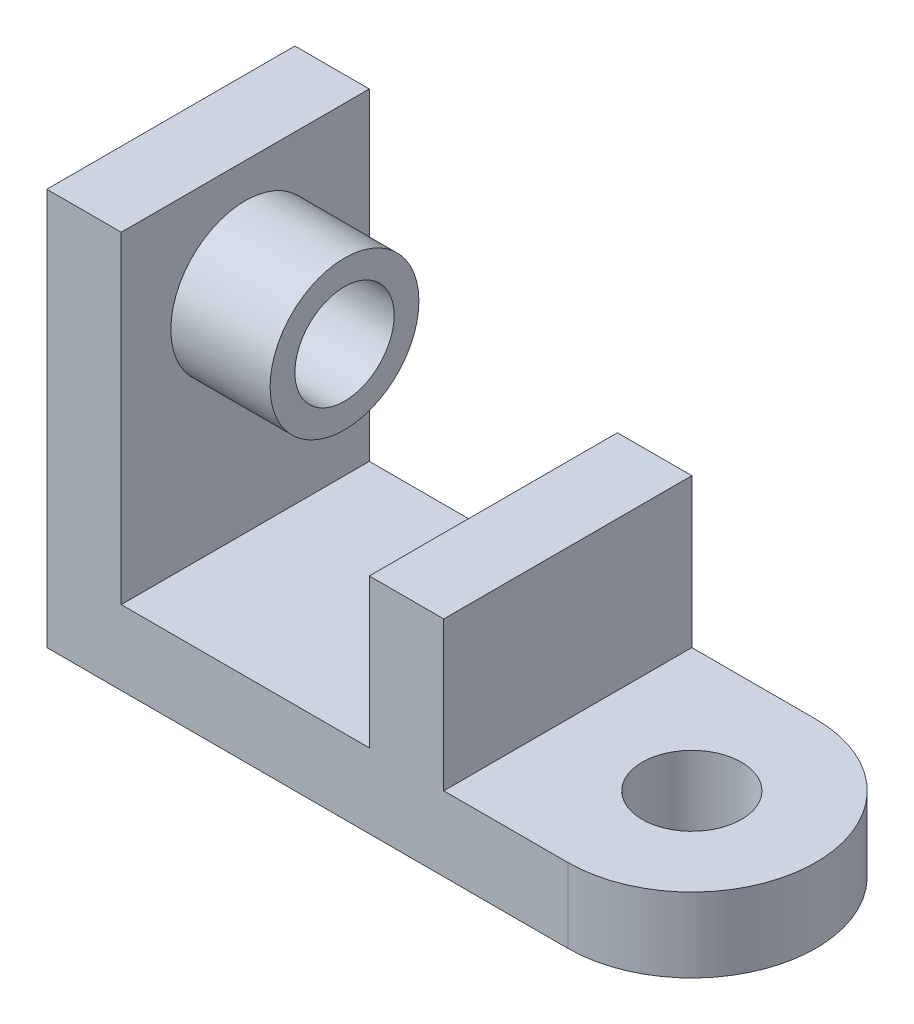
ISO-10303-21;
HEADER;
FILE_DESCRIPTION(('STEP AP214'),'2;1');
FILE_NAME('part.step','',(''),(''),'','','');
FILE_SCHEMA(('AUTOMOTIVE_DESIGN { 1 0 10303 214 1 1 1 1 }'));
ENDSEC;
DATA;
#1=APPLICATION_CONTEXT('core data for automotive mechanical design processes');
#2=APPLICATION_PROTOCOL_DEFINITION('international standard','automotive_design',2000,#1);
#3=PRODUCT_CONTEXT('',#1,'mechanical');
#4=PRODUCT('Part','Part','',(#3));
#5=PRODUCT_RELATED_PRODUCT_CATEGORY('part','',(#4));
#6=PRODUCT_DEFINITION_FORMATION('','',#4);
#7=PRODUCT_DEFINITION_CONTEXT('part definition',#1,'design');
#8=PRODUCT_DEFINITION('design','',#6,#7);
#9=PRODUCT_DEFINITION_SHAPE('','',#8);
#10=(LENGTH_UNIT() NAMED_UNIT(*) SI_UNIT(.MILLI.,.METRE.));
#11=(NAMED_UNIT(*) PLANE_ANGLE_UNIT() SI_UNIT($,.RADIAN.));
#12=(NAMED_UNIT(*) SI_UNIT($,.STERADIAN.) SOLID_ANGLE_UNIT());
#13=UNCERTAINTY_MEASURE_WITH_UNIT(LENGTH_MEASURE(1.E-05),#10,'distance_accuracy_value','');
#14=(GEOMETRIC_REPRESENTATION_CONTEXT(3) GLOBAL_UNCERTAINTY_ASSIGNED_CONTEXT((#13)) GLOBAL_UNIT_ASSIGNED_CONTEXT((#10,
#11,#12)) REPRESENTATION_CONTEXT('',''));
#15=CARTESIAN_POINT('',(0.,0.,0.));
#16=DIRECTION('',(0.,0.,1.));
#17=DIRECTION('',(1.,0.,0.));
#18=AXIS2_PLACEMENT_3D('',#15,#16,#17);
#19=CARTESIAN_POINT('',(40.,15.,0.));
#20=DIRECTION('',(0.,1.,0.));
#21=DIRECTION('',(0.,0.,1.));
#22=AXIS2_PLACEMENT_3D('',#19,#20,#21);
#23=PLANE('',#22);
#24=DIRECTION('',(1.,0.,0.));
#25=VECTOR('',#24,1.);
#26=CARTESIAN_POINT('',(-65.,15.,25.));
#27=LINE('',#26,#25);
#28=CARTESIAN_POINT('',(-50.,15.,25.));
#29=VERTEX_POINT('',#28);
#30=CARTESIAN_POINT('',(0.,15.,25.));
#31=VERTEX_POINT('',#30);
#32=EDGE_CURVE('E175',#29,#31,#27,.T.);
#33=ORIENTED_EDGE('',*,*,#32,.T.);
#34=DIRECTION('',(0.,0.,1.));
#35=VECTOR('',#34,1.);
#36=CARTESIAN_POINT('',(0.,15.,25.));
#37=LINE('',#36,#35);
#38=CARTESIAN_POINT('',(0.,15.,-25.));
#39=VERTEX_POINT('',#38);
#40=EDGE_CURVE('E223',#39,#31,#37,.T.);
#41=ORIENTED_EDGE('',*,*,#40,.F.);
#42=DIRECTION('',(-1.,0.,0.));
#43=VECTOR('',#42,1.);
#44=CARTESIAN_POINT('',(-65.,15.,-25.));
#45=LINE('',#44,#43);
#46=CARTESIAN_POINT('',(-50.,15.,-25.));
#47=VERTEX_POINT('',#46);
#48=EDGE_CURVE('E141',#39,#47,#45,.T.);
#49=ORIENTED_EDGE('',*,*,#48,.T.);
#50=DIRECTION('',(0.,0.,-1.));
#51=VECTOR('',#50,1.);
#52=CARTESIAN_POINT('',(-50.,15.,25.));
#53=LINE('',#52,#51);
#54=EDGE_CURVE('E65',#29,#47,#53,.T.);
#55=ORIENTED_EDGE('',*,*,#54,.F.);
#56=EDGE_LOOP('',(#33,#41,#49,#55));
#57=FACE_BOUND('',#56,.T.);
#58=ADVANCED_FACE('F41',(#57),#23,.T.);
#59=CARTESIAN_POINT('',(40.,15.,0.));
#60=DIRECTION('',(0.,1.,0.));
#61=DIRECTION('',(0.,0.,1.));
#62=AXIS2_PLACEMENT_3D('',#59,#60,#61);
#63=CIRCLE('',#62,10.);
#64=CARTESIAN_POINT('',(40.,15.,10.));
#65=VERTEX_POINT('',#64);
#66=EDGE_CURVE('E230',#65,#65,#63,.T.);
#67=ORIENTED_EDGE('',*,*,#66,.F.);
#68=EDGE_LOOP('',(#67));
#69=FACE_BOUND('',#68,.T.);
#70=CARTESIAN_POINT('',(40.,15.,-25.));
#71=VERTEX_POINT('',#70);
#72=CARTESIAN_POINT('',(15.,15.,-25.));
#73=VERTEX_POINT('',#72);
#74=EDGE_CURVE('E180',#71,#73,#45,.T.);
#75=ORIENTED_EDGE('',*,*,#74,.T.);
#76=DIRECTION('',(0.,0.,-1.));
#77=VECTOR('',#76,1.);
#78=CARTESIAN_POINT('',(15.,15.,-25.));
#79=LINE('',#78,#77);
#80=CARTESIAN_POINT('',(15.,15.,25.));
#81=VERTEX_POINT('',#80);
#82=EDGE_CURVE('E137',#81,#73,#79,.T.);
#83=ORIENTED_EDGE('',*,*,#82,.F.);
#84=CARTESIAN_POINT('',(40.,15.,25.));
#85=VERTEX_POINT('',#84);
#86=EDGE_CURVE('E179',#81,#85,#27,.T.);
#87=ORIENTED_EDGE('',*,*,#86,.T.);
#88=CARTESIAN_POINT('',(40.,15.,0.));
#89=DIRECTION('',(0.,1.,0.));
#90=DIRECTION('',(0.,0.,1.));
#91=AXIS2_PLACEMENT_3D('',#88,#89,#90);
#92=CIRCLE('',#91,25.);
#93=EDGE_CURVE('E178',#85,#71,#92,.T.);
#94=ORIENTED_EDGE('',*,*,#93,.T.);
#95=EDGE_LOOP('',(#75,#83,#87,#94));
#96=FACE_BOUND('',#95,.T.);
#97=ADVANCED_FACE('F217',(#69,#96),#23,.T.);
#98=CARTESIAN_POINT('',(-65.,15.,25.));
#99=DIRECTION('',(1.,0.,0.));
#100=DIRECTION('',(0.,0.,-1.));
#101=AXIS2_PLACEMENT_3D('',#98,#99,#100);
#102=PLANE('',#101);
#103=DIRECTION('',(0.,0.,1.));
#104=VECTOR('',#103,1.);
#105=CARTESIAN_POINT('',(-65.,0.,25.));
#106=LINE('',#105,#104);
#107=CARTESIAN_POINT('',(-65.,0.,-25.));
#108=VERTEX_POINT('',#107);
#109=CARTESIAN_POINT('',(-65.,0.,25.));
#110=VERTEX_POINT('',#109);
#111=EDGE_CURVE('E172',#108,#110,#106,.T.);
#112=ORIENTED_EDGE('',*,*,#111,.T.);
#113=DIRECTION('',(0.,-1.,0.));
#114=VECTOR('',#113,1.);
#115=CARTESIAN_POINT('',(-65.,15.,25.));
#116=LINE('',#115,#114);
#117=CARTESIAN_POINT('',(-65.,80.,25.));
#118=VERTEX_POINT('',#117);
#119=EDGE_CURVE('E47',#118,#110,#116,.T.);
#120=ORIENTED_EDGE('',*,*,#119,.F.);
#121=DIRECTION('',(0.,0.,1.));
#122=VECTOR('',#121,1.);
#123=CARTESIAN_POINT('',(-65.,80.,25.));
#124=LINE('',#123,#122);
#125=CARTESIAN_POINT('',(-65.,80.,-25.));
#126=VERTEX_POINT('',#125);
#127=EDGE_CURVE('E160',#126,#118,#124,.T.);
#128=ORIENTED_EDGE('',*,*,#127,.F.);
#129=DIRECTION('',(0.,-1.,0.));
#130=VECTOR('',#129,1.);
#131=CARTESIAN_POINT('',(-65.,15.,-25.));
#132=LINE('',#131,#130);
#133=EDGE_CURVE('E185',#126,#108,#132,.T.);
#134=ORIENTED_EDGE('',*,*,#133,.T.);
#135=EDGE_LOOP('',(#112,#120,#128,#134));
#136=FACE_BOUND('',#135,.T.);
#137=ADVANCED_FACE('F43',(#136),#102,.F.);
#138=CARTESIAN_POINT('',(-65.,15.,25.));
#139=DIRECTION('',(0.,0.,-1.));
#140=DIRECTION('',(-1.,0.,0.));
#141=AXIS2_PLACEMENT_3D('',#138,#139,#140);
#142=PLANE('',#141);
#143=DIRECTION('',(1.,0.,0.));
#144=VECTOR('',#143,1.);
#145=CARTESIAN_POINT('',(-65.,0.,25.));
#146=LINE('',#145,#144);
#147=CARTESIAN_POINT('',(40.,0.,25.));
#148=VERTEX_POINT('',#147);
#149=EDGE_CURVE('E183',#110,#148,#146,.T.);
#150=ORIENTED_EDGE('',*,*,#149,.T.);
#151=DIRECTION('',(0.,-1.,0.));
#152=VECTOR('',#151,1.);
#153=CARTESIAN_POINT('',(40.,15.,25.));
#154=LINE('',#153,#152);
#155=EDGE_CURVE('E198',#85,#148,#154,.T.);
#156=ORIENTED_EDGE('',*,*,#155,.F.);
#157=ORIENTED_EDGE('',*,*,#86,.F.);
#158=DIRECTION('',(0.,-1.,0.));
#159=VECTOR('',#158,1.);
#160=CARTESIAN_POINT('',(15.,45.,25.));
#161=LINE('',#160,#159);
#162=CARTESIAN_POINT('',(15.,45.,25.));
#163=VERTEX_POINT('',#162);
#164=EDGE_CURVE('E57',#163,#81,#161,.T.);
#165=ORIENTED_EDGE('',*,*,#164,.F.);
#166=DIRECTION('',(1.,0.,0.));
#167=VECTOR('',#166,1.);
#168=CARTESIAN_POINT('',(15.,45.,25.));
#169=LINE('',#168,#167);
#170=CARTESIAN_POINT('',(0.,45.,25.));
#171=VERTEX_POINT('',#170);
#172=EDGE_CURVE('E129',#171,#163,#169,.T.);
#173=ORIENTED_EDGE('',*,*,#172,.F.);
#174=DIRECTION('',(0.,-1.,0.));
#175=VECTOR('',#174,1.);
#176=CARTESIAN_POINT('',(0.,45.,25.));
#177=LINE('',#176,#175);
#178=EDGE_CURVE('E127',#171,#31,#177,.T.);
#179=ORIENTED_EDGE('',*,*,#178,.T.);
#180=ORIENTED_EDGE('',*,*,#32,.F.);
#181=DIRECTION('',(0.,-1.,0.));
#182=VECTOR('',#181,1.);
#183=CARTESIAN_POINT('',(-50.,80.,25.));
#184=LINE('',#183,#182);
#185=CARTESIAN_POINT('',(-50.,80.,25.));
#186=VERTEX_POINT('',#185);
#187=EDGE_CURVE('E168',#186,#29,#184,.T.);
#188=ORIENTED_EDGE('',*,*,#187,.F.);
#189=DIRECTION('',(1.,0.,0.));
#190=VECTOR('',#189,1.);
#191=CARTESIAN_POINT('',(-65.,80.,25.));
#192=LINE('',#191,#190);
#193=EDGE_CURVE('E159',#118,#186,#192,.T.);
#194=ORIENTED_EDGE('',*,*,#193,.F.);
#195=ORIENTED_EDGE('',*,*,#119,.T.);
#196=EDGE_LOOP('',(#150,#156,#157,#165,#173,#179,#180,#188,#194,#195));
#197=FACE_BOUND('',#196,.T.);
#198=ADVANCED_FACE('F203',(#197),#142,.F.);
#199=CARTESIAN_POINT('',(40.,15.,0.));
#200=DIRECTION('',(0.,-1.,0.));
#201=DIRECTION('',(0.,0.,-1.));
#202=AXIS2_PLACEMENT_3D('',#199,#200,#201);
#203=CYLINDRICAL_SURFACE('',#202,25.);
#204=CARTESIAN_POINT('',(40.,0.,0.));
#205=DIRECTION('',(0.,1.,0.));
#206=DIRECTION('',(0.,0.,1.));
#207=AXIS2_PLACEMENT_3D('',#204,#205,#206);
#208=CIRCLE('',#207,25.);
#209=CARTESIAN_POINT('',(40.,0.,-25.));
#210=VERTEX_POINT('',#209);
#211=EDGE_CURVE('E189',#148,#210,#208,.T.);
#212=ORIENTED_EDGE('',*,*,#211,.T.);
#213=DIRECTION('',(0.,-1.,0.));
#214=VECTOR('',#213,1.);
#215=CARTESIAN_POINT('',(40.,15.,-25.));
#216=LINE('',#215,#214);
#217=EDGE_CURVE('E192',#71,#210,#216,.T.);
#218=ORIENTED_EDGE('',*,*,#217,.F.);
#219=ORIENTED_EDGE('',*,*,#93,.F.);
#220=ORIENTED_EDGE('',*,*,#155,.T.);
#221=EDGE_LOOP('',(#212,#218,#219,#220));
#222=FACE_BOUND('',#221,.T.);
#223=ADVANCED_FACE('F213',(#222),#203,.T.);
#224=CARTESIAN_POINT('',(-65.,15.,-25.));
#225=DIRECTION('',(0.,0.,1.));
#226=DIRECTION('',(1.,0.,0.));
#227=AXIS2_PLACEMENT_3D('',#224,#225,#226);
#228=PLANE('',#227);
#229=DIRECTION('',(-1.,0.,0.));
#230=VECTOR('',#229,1.);
#231=CARTESIAN_POINT('',(-65.,0.,-25.));
#232=LINE('',#231,#230);
#233=EDGE_CURVE('E190',#210,#108,#232,.T.);
#234=ORIENTED_EDGE('',*,*,#233,.T.);
#235=ORIENTED_EDGE('',*,*,#133,.F.);
#236=DIRECTION('',(-1.,0.,0.));
#237=VECTOR('',#236,1.);
#238=CARTESIAN_POINT('',(-65.,80.,-25.));
#239=LINE('',#238,#237);
#240=CARTESIAN_POINT('',(-50.,80.,-25.));
#241=VERTEX_POINT('',#240);
#242=EDGE_CURVE('E163',#241,#126,#239,.T.);
#243=ORIENTED_EDGE('',*,*,#242,.F.);
#244=DIRECTION('',(0.,-1.,0.));
#245=VECTOR('',#244,1.);
#246=CARTESIAN_POINT('',(-50.,80.,-25.));
#247=LINE('',#246,#245);
#248=EDGE_CURVE('E170',#241,#47,#247,.T.);
#249=ORIENTED_EDGE('',*,*,#248,.T.);
#250=ORIENTED_EDGE('',*,*,#48,.F.);
#251=DIRECTION('',(0.,-1.,0.));
#252=VECTOR('',#251,1.);
#253=CARTESIAN_POINT('',(0.,45.,-25.));
#254=LINE('',#253,#252);
#255=CARTESIAN_POINT('',(0.,45.,-25.));
#256=VERTEX_POINT('',#255);
#257=EDGE_CURVE('E122',#256,#39,#254,.T.);
#258=ORIENTED_EDGE('',*,*,#257,.F.);
#259=DIRECTION('',(-1.,0.,0.));
#260=VECTOR('',#259,1.);
#261=CARTESIAN_POINT('',(0.,45.,-25.));
#262=LINE('',#261,#260);
#263=CARTESIAN_POINT('',(15.,45.,-25.));
#264=VERTEX_POINT('',#263);
#265=EDGE_CURVE('E128',#264,#256,#262,.T.);
#266=ORIENTED_EDGE('',*,*,#265,.F.);
#267=DIRECTION('',(0.,-1.,0.));
#268=VECTOR('',#267,1.);
#269=CARTESIAN_POINT('',(15.,45.,-25.));
#270=LINE('',#269,#268);
#271=EDGE_CURVE('E216',#264,#73,#270,.T.);
#272=ORIENTED_EDGE('',*,*,#271,.T.);
#273=ORIENTED_EDGE('',*,*,#74,.F.);
#274=ORIENTED_EDGE('',*,*,#217,.T.);
#275=EDGE_LOOP('',(#234,#235,#243,#249,#250,#258,#266,#272,#273,#274));
#276=FACE_BOUND('',#275,.T.);
#277=ADVANCED_FACE('F143',(#276),#228,.F.);
#278=CARTESIAN_POINT('',(40.,0.,0.));
#279=DIRECTION('',(0.,1.,0.));
#280=DIRECTION('',(0.,0.,1.));
#281=AXIS2_PLACEMENT_3D('',#278,#279,#280);
#282=PLANE('',#281);
#283=CARTESIAN_POINT('',(40.,0.,0.));
#284=DIRECTION('',(0.,1.,0.));
#285=DIRECTION('',(0.,0.,1.));
#286=AXIS2_PLACEMENT_3D('',#283,#284,#285);
#287=CIRCLE('',#286,10.);
#288=CARTESIAN_POINT('',(40.,0.,10.));
#289=VERTEX_POINT('',#288);
#290=EDGE_CURVE('E229',#289,#289,#287,.T.);
#291=ORIENTED_EDGE('',*,*,#290,.T.);
#292=EDGE_LOOP('',(#291));
#293=FACE_BOUND('',#292,.T.);
#294=ORIENTED_EDGE('',*,*,#111,.F.);
#295=ORIENTED_EDGE('',*,*,#233,.F.);
#296=ORIENTED_EDGE('',*,*,#211,.F.);
#297=ORIENTED_EDGE('',*,*,#149,.F.);
#298=EDGE_LOOP('',(#294,#295,#296,#297));
#299=FACE_BOUND('',#298,.T.);
#300=ADVANCED_FACE('F207',(#293,#299),#282,.F.);
#301=CARTESIAN_POINT('',(-50.,80.,25.));
#302=DIRECTION('',(-1.,0.,0.));
#303=DIRECTION('',(0.,0.,1.));
#304=AXIS2_PLACEMENT_3D('',#301,#302,#303);
#305=PLANE('',#304);
#306=CARTESIAN_POINT('',(-50.,58.,0.));
#307=DIRECTION('',(-1.,0.,0.));
#308=DIRECTION('',(0.,0.,1.));
#309=AXIS2_PLACEMENT_3D('',#306,#307,#308);
#310=CIRCLE('',#309,15.);
#311=CARTESIAN_POINT('',(-50.,58.,15.));
#312=VERTEX_POINT('',#311);
#313=EDGE_CURVE('E11',#312,#312,#310,.F.);
#314=ORIENTED_EDGE('',*,*,#313,.F.);
#315=EDGE_LOOP('',(#314));
#316=FACE_BOUND('',#315,.T.);
#317=ORIENTED_EDGE('',*,*,#54,.T.);
#318=ORIENTED_EDGE('',*,*,#248,.F.);
#319=DIRECTION('',(0.,0.,-1.));
#320=VECTOR('',#319,1.);
#321=CARTESIAN_POINT('',(-50.,80.,25.));
#322=LINE('',#321,#320);
#323=EDGE_CURVE('E165',#186,#241,#322,.T.);
#324=ORIENTED_EDGE('',*,*,#323,.F.);
#325=ORIENTED_EDGE('',*,*,#187,.T.);
#326=EDGE_LOOP('',(#317,#318,#324,#325));
#327=FACE_BOUND('',#326,.T.);
#328=ADVANCED_FACE('F250',(#316,#327),#305,.F.);
#329=CARTESIAN_POINT('',(0.,80.,0.));
#330=DIRECTION('',(0.,-1.,0.));
#331=DIRECTION('',(0.,0.,-1.));
#332=AXIS2_PLACEMENT_3D('',#329,#330,#331);
#333=PLANE('',#332);
#334=ORIENTED_EDGE('',*,*,#127,.T.);
#335=ORIENTED_EDGE('',*,*,#193,.T.);
#336=ORIENTED_EDGE('',*,*,#323,.T.);
#337=ORIENTED_EDGE('',*,*,#242,.T.);
#338=EDGE_LOOP('',(#334,#335,#336,#337));
#339=FACE_BOUND('',#338,.T.);
#340=ADVANCED_FACE('F333',(#339),#333,.F.);
#341=CARTESIAN_POINT('',(-30.,58.,0.));
#342=DIRECTION('',(-1.,0.,0.));
#343=DIRECTION('',(0.,0.,1.));
#344=AXIS2_PLACEMENT_3D('',#341,#342,#343);
#345=CYLINDRICAL_SURFACE('',#344,15.);
#346=CARTESIAN_POINT('',(-30.,58.,0.));
#347=DIRECTION('',(1.,0.,0.));
#348=DIRECTION('',(0.,0.,-1.));
#349=AXIS2_PLACEMENT_3D('',#346,#347,#348);
#350=CIRCLE('',#349,15.);
#351=CARTESIAN_POINT('',(-30.,58.,-15.));
#352=VERTEX_POINT('',#351);
#353=EDGE_CURVE('E153',#352,#352,#350,.T.);
#354=ORIENTED_EDGE('',*,*,#353,.F.);
#355=EDGE_LOOP('',(#354));
#356=FACE_BOUND('',#355,.T.);
#357=ORIENTED_EDGE('',*,*,#313,.T.);
#358=EDGE_LOOP('',(#357));
#359=FACE_BOUND('',#358,.T.);
#360=ADVANCED_FACE('F345',(#356,#359),#345,.T.);
#361=CARTESIAN_POINT('',(-30.,58.,0.));
#362=DIRECTION('',(1.,0.,0.));
#363=DIRECTION('',(0.,0.,-1.));
#364=AXIS2_PLACEMENT_3D('',#361,#362,#363);
#365=PLANE('',#364);
#366=CARTESIAN_POINT('',(-30.,58.,0.));
#367=DIRECTION('',(1.,0.,0.));
#368=DIRECTION('',(0.,0.,-1.));
#369=AXIS2_PLACEMENT_3D('',#366,#367,#368);
#370=CIRCLE('',#369,10.);
#371=CARTESIAN_POINT('',(-30.,58.,-10.));
#372=VERTEX_POINT('',#371);
#373=EDGE_CURVE('E145',#372,#372,#370,.T.);
#374=ORIENTED_EDGE('',*,*,#373,.F.);
#375=EDGE_LOOP('',(#374));
#376=FACE_BOUND('',#375,.T.);
#377=ORIENTED_EDGE('',*,*,#353,.T.);
#378=EDGE_LOOP('',(#377));
#379=FACE_BOUND('',#378,.T.);
#380=ADVANCED_FACE('F354',(#376,#379),#365,.T.);
#381=CARTESIAN_POINT('',(-50.,58.,0.));
#382=DIRECTION('',(1.,0.,0.));
#383=DIRECTION('',(0.,0.,-1.));
#384=AXIS2_PLACEMENT_3D('',#381,#382,#383);
#385=CYLINDRICAL_SURFACE('',#384,10.);
#386=CARTESIAN_POINT('',(-50.,58.,0.));
#387=DIRECTION('',(1.,0.,0.));
#388=DIRECTION('',(0.,0.,-1.));
#389=AXIS2_PLACEMENT_3D('',#386,#387,#388);
#390=CIRCLE('',#389,10.);
#391=CARTESIAN_POINT('',(-50.,58.,-10.));
#392=VERTEX_POINT('',#391);
#393=EDGE_CURVE('E150',#392,#392,#390,.T.);
#394=ORIENTED_EDGE('',*,*,#393,.F.);
#395=EDGE_LOOP('',(#394));
#396=FACE_BOUND('',#395,.T.);
#397=ORIENTED_EDGE('',*,*,#373,.T.);
#398=EDGE_LOOP('',(#397));
#399=FACE_BOUND('',#398,.T.);
#400=ADVANCED_FACE('F362',(#396,#399),#385,.F.);
#401=CARTESIAN_POINT('',(-50.,58.,0.));
#402=DIRECTION('',(1.,0.,0.));
#403=DIRECTION('',(0.,0.,-1.));
#404=AXIS2_PLACEMENT_3D('',#401,#402,#403);
#405=PLANE('',#404);
#406=ORIENTED_EDGE('',*,*,#393,.T.);
#407=EDGE_LOOP('',(#406));
#408=FACE_BOUND('',#407,.T.);
#409=ADVANCED_FACE('F273',(#408),#405,.T.);
#410=CARTESIAN_POINT('',(0.,45.,25.));
#411=DIRECTION('',(1.,0.,0.));
#412=DIRECTION('',(0.,0.,-1.));
#413=AXIS2_PLACEMENT_3D('',#410,#411,#412);
#414=PLANE('',#413);
#415=ORIENTED_EDGE('',*,*,#40,.T.);
#416=ORIENTED_EDGE('',*,*,#178,.F.);
#417=DIRECTION('',(0.,0.,1.));
#418=VECTOR('',#417,1.);
#419=CARTESIAN_POINT('',(0.,45.,25.));
#420=LINE('',#419,#418);
#421=EDGE_CURVE('E120',#256,#171,#420,.T.);
#422=ORIENTED_EDGE('',*,*,#421,.F.);
#423=ORIENTED_EDGE('',*,*,#257,.T.);
#424=EDGE_LOOP('',(#415,#416,#422,#423));
#425=FACE_BOUND('',#424,.T.);
#426=ADVANCED_FACE('F123',(#425),#414,.F.);
#427=CARTESIAN_POINT('',(15.,45.,-25.));
#428=DIRECTION('',(-1.,0.,0.));
#429=DIRECTION('',(0.,0.,1.));
#430=AXIS2_PLACEMENT_3D('',#427,#428,#429);
#431=PLANE('',#430);
#432=ORIENTED_EDGE('',*,*,#82,.T.);
#433=ORIENTED_EDGE('',*,*,#271,.F.);
#434=DIRECTION('',(0.,0.,-1.));
#435=VECTOR('',#434,1.);
#436=CARTESIAN_POINT('',(15.,45.,-25.));
#437=LINE('',#436,#435);
#438=EDGE_CURVE('E135',#163,#264,#437,.T.);
#439=ORIENTED_EDGE('',*,*,#438,.F.);
#440=ORIENTED_EDGE('',*,*,#164,.T.);
#441=EDGE_LOOP('',(#432,#433,#439,#440));
#442=FACE_BOUND('',#441,.T.);
#443=ADVANCED_FACE('F219',(#442),#431,.F.);
#444=CARTESIAN_POINT('',(0.,45.,0.));
#445=DIRECTION('',(0.,-1.,0.));
#446=DIRECTION('',(0.,0.,-1.));
#447=AXIS2_PLACEMENT_3D('',#444,#445,#446);
#448=PLANE('',#447);
#449=ORIENTED_EDGE('',*,*,#265,.T.);
#450=ORIENTED_EDGE('',*,*,#421,.T.);
#451=ORIENTED_EDGE('',*,*,#172,.T.);
#452=ORIENTED_EDGE('',*,*,#438,.T.);
#453=EDGE_LOOP('',(#449,#450,#451,#452));
#454=FACE_BOUND('',#453,.T.);
#455=ADVANCED_FACE('F132',(#454),#448,.F.);
#456=CARTESIAN_POINT('',(40.,0.,0.));
#457=DIRECTION('',(0.,1.,0.));
#458=DIRECTION('',(0.,0.,1.));
#459=AXIS2_PLACEMENT_3D('',#456,#457,#458);
#460=CYLINDRICAL_SURFACE('',#459,10.);
#461=ORIENTED_EDGE('',*,*,#290,.F.);
#462=EDGE_LOOP('',(#461));
#463=FACE_BOUND('',#462,.T.);
#464=ORIENTED_EDGE('',*,*,#66,.T.);
#465=EDGE_LOOP('',(#464));
#466=FACE_BOUND('',#465,.T.);
#467=ADVANCED_FACE('F240',(#463,#466),#460,.F.);
#468=CLOSED_SHELL('',(#58,#97,#137,#198,#223,#277,#300,#328,#340,#360,#380,#400,#409,#426,#443,
#455,#467));
#469=MANIFOLD_SOLID_BREP('B2',#468);
#470=ADVANCED_BREP_SHAPE_REPRESENTATION('',(#18,#469),#14);
#471=SHAPE_DEFINITION_REPRESENTATION(#9,#470);
ENDSEC;
END-ISO-10303-21;
